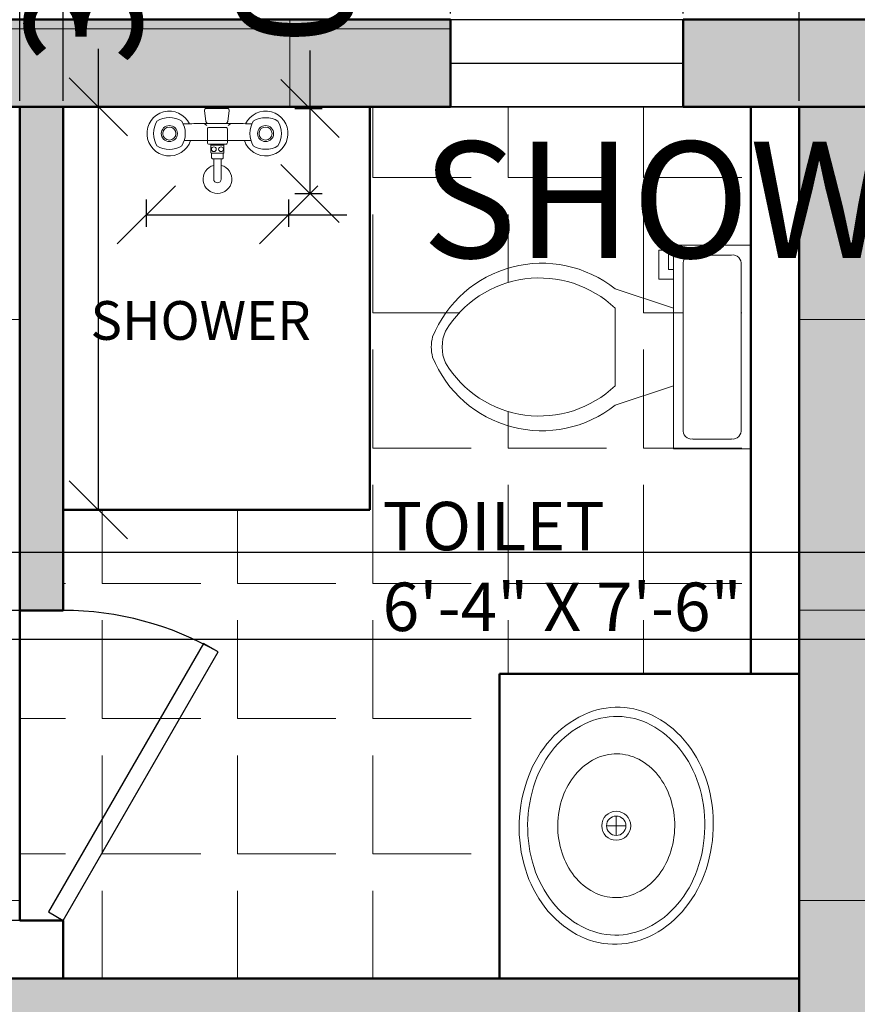
# Model space of a CAD drawing. Units: inches. Extents: x 2371 to 3019, y 129 to 700.
# Tile 6 of 14: x 2492 to 2579, y 529 to 631. Entities that reach past the tile are written whole.
import ezdxf

# ---------------------------------------------------------------- set-up
doc = ezdxf.new("R2010")
doc.units = ezdxf.units.IN
for name, color, linetype, lineweight in [('A-ANNO-DIMS', 2, 'Continuous', 18), ('A-AREA-IDEN', 7, 'Continuous', 25), ('A-DOOR', 4, 'Continuous', 25), ('A-FLOR-FIXT', 8, 'Continuous', 18), ('A-FLOR-PATT', 252, 'Continuous', 13), ('A-FURN', 8, 'Continuous', 18), ('A-GLAZ', 4, 'Continuous', 25), ('A-WALL', 7, 'Continuous', 50), ('A-WALL-PATT', 8, 'Continuous', 13)]:
    doc.layers.add(name, color=color, linetype=linetype, lineweight=lineweight)
doc.styles.get("Standard").update_dxf_attribs({"font": 'arial.ttf'})
doc.dimstyles.new('ISO-25', dxfattribs={"dimtxt": 12, "dimasz": 6, "dimexe": 1.25, "dimexo": 0.625, "dimtad": 0, "dimdec": 1, "dimlunit": 3, "dimtxsty": 'Standard', "dimblk": 'OBLIQUE', "dimblk1": 'ORIGIN2', "dimblk2": 'OBLIQUE', "dimcen": 2.5, "dimadec": 0, "dimazin": 0, "dimtfac": 1, "dimtdec": 1, "dimtmove": 0, "dimatfit": 3, "dimldrblk": 'OBLIQUE', "dimfxl": 1, "dimarcsym": 0})

# ---------------------------------------------------------------- blocks, each defined once
blk = doc.blocks.new('*U3')
for p, q in [((0, 0), (0, -6)), ((-32, 0), (-32, -6))]:
    blk.add_line(p, q)
blk.add_lwpolyline([(0, 0), (-27.71, 16), (-28.59, 14.48), (-0.88, -1.52)], close=True)
blk.add_arc((0, 0), 32, 150, 180)
blk = doc.blocks.new('Toilet - top')
for p, q in [((9.5, -6), (9.5, -2)), ((-8, -8.5), (-8, -8)), ((-7, -8), (-7, -9.5)), ((-4, -8), (-6, -14)), ((4, -8), (6, -14)), ((-10, -8.5), (-8, -8.5)), ((-10, -9.5), (-10, -8.5)), ((-7, -9.5), (-10, -9.5)), ((4, -14), (-4, -14))]:
    blk.add_line(p, q)
blk.add_lwpolyline([(10.5, -8), (10.5, 0), (-10.5, 0), (-10.5, -8)], close=True)
for points in [[(8.5, -1), (-8.5, -1)], [(-9.5, -2), (-9.5, -6)], [(-8.5, -7), (8.5, -7)]]:
    blk.add_lwpolyline(points)
for centre, radius, start, end in [((-8.62, -1.88), 0.884, 81.8699, 188.1301), ((8.62, -1.88), 0.884, 351.8699, 98.1301), ((-8.62, -6.12), 0.884, 171.8699, 278.1301), ((8.62, -6.12), 0.884, 261.8699, 8.1301), ((3.52, -21.58), 12.17, 141.4691, 247.9714), ((4.2, -21.82), 11.33, 136.3677, 238.9468), ((-3.52, -21.58), 12.17, 292.0284, 38.5307), ((-4.2, -21.82), 11.33, 301.053, 43.6321), ((0, -27.88), 4, 245.7318, 294.2682), ((0, -29), 4, 254.8605, 285.1395)]:
    blk.add_arc(centre, radius, start, end)
blk = doc.blocks.new('Sink - Oval top')
for p, q in [((-1, 0), (1, 0)), ((0, 1), (0, -1))]:
    blk.add_line(p, q)
for points in [[(-12.23, 0.39, 0.117634), (-11.46, -3.36, 0.104469), (-8.88, -6.8, 0.090016), (-5.08, -9.07, 0.08192), (-0.32, -10.02, 0.08192), (4.49, -9.38, 0.090016), (8.42, -7.36, 0.104469), (11.22, -4.09, 0.117634), (12.23, -0.39, 0.117634), (11.46, 3.36, 0.104469), (8.88, 6.8, 0.090016), (5.08, 9.07, 0.08192), (0.32, 10.02, 0.08192), (-4.49, 9.38, 0.090016), (-8.42, 7.36, 0.104469), (-11.22, 4.09, 0.117634)], [(-11.29, 0.16, 0.118622), (-10.52, -3.25, 0.104678), (-8.07, -6.36, 0.089562), (-4.54, -8.37, 0.081185), (-0.13, -9.15, 0.081185), (4.3, -8.49, 0.089562), (7.89, -6.58, 0.104678), (10.42, -3.55, 0.118622), (11.29, -0.16, 0.118622), (10.52, 3.25, 0.104678), (8.07, 6.36, 0.089562), (4.54, 8.37, 0.081185), (0.13, 9.15, 0.081185), (-4.3, 8.49, 0.089562), (-7.89, 6.58, 0.104678), (-10.42, 3.55, 0.118622)], [(-7.42, 0.08, 0.118283), (-6.91, -2.17, 0.104607), (-5.29, -4.21, 0.089718), (-2.97, -5.53, 0.081436), (-0.07, -6.04, 0.081436), (2.84, -5.59, 0.089718), (5.2, -4.33, 0.104607), (6.86, -2.32, 0.118283), (7.42, -0.08, 0.118283), (6.91, 2.17, 0.104607), (5.29, 4.21, 0.089718), (2.97, 5.53, 0.081436), (0.07, 6.04, 0.081436), (-2.84, 5.59, 0.089718), (-5.2, 4.33, 0.104607), (-6.86, 2.32, 0.118283)]]:
    blk.add_lwpolyline(points, format="xyb", close=True)
for radius in [1.5, 1]:
    blk.add_circle((0, 0), radius)
blk = doc.blocks.new('_Oblique')
at = {"color": 0, "linetype": 'ByBlock', "lineweight": -2}
blk.add_line((-0.5, -0.5), (0.5, 0.5), dxfattribs=at)
blk = doc.blocks.new('*D14')
at = {"layer": 'A-ANNO-DIMS', "color": 0, "lineweight": -2, "transparency": 16777216}
for p, q in [((2407.11, 631.6), (2407.11, 649.37)), ((2923.11, 631.6), (2923.11, 649.37)), ((2407.11, 648.12), (2643.63, 648.12)), ((2923.11, 648.12), (2686.58, 648.12))]:
    blk.add_line(p, q, dxfattribs=at)
at = {"layer": 'Defpoints', "color": 0, "lineweight": 25, "transparency": 16777216}
for p in [(2923.11, 648.12), (2407.11, 630.98), (2923.11, 630.98)]:
    blk.add_point(p, dxfattribs=at)
at = {"layer": 'A-ANNO-DIMS', "color": 0, "lineweight": -2, "transparency": 16777216, "xscale": 6, "yscale": 6, "zscale": 6, "rotation": 180}
blk.add_blockref('_Oblique', (2407.11, 648.12), dxfattribs=at)
at = {"layer": 'A-ANNO-DIMS', "color": 0, "lineweight": -2, "transparency": 16777216, "xscale": 6, "yscale": 6, "zscale": 6}
blk.add_blockref('_Oblique', (2923.11, 648.12), dxfattribs=at)
at = {"layer": 'A-ANNO-DIMS', "color": 0, "transparency": 16777216, "insert": (2665.11, 648.12), "char_height": 12, "width": 20.8486, "attachment_point": 5}
blk.add_mtext('43\'-0"', dxfattribs=at)
blk = doc.blocks.new('_Origin2')
at = {"color": 0, "linetype": 'ByBlock', "lineweight": -2}
blk.add_line((-0.5, 0), (-1, 0), dxfattribs=at)
for radius in [0.5, 0.25]:
    blk.add_circle((0, 0), radius, dxfattribs=at)
blk = doc.blocks.new('SHOWER-MIXER')
for points in [[(2511.46, 620.27), (2511.32, 620.45), (2511.19, 621.61, -0.472691), (2511.38, 621.8)], [(2513.47, 620.27), (2513.61, 620.45), (2513.75, 621.61, 0.472691), (2513.56, 621.8)], [(2506.28, 620.5, 0.281574), (2506.28, 617.95, 3.55146)], [(2508.84, 620.5, 0.281574), (2506.28, 620.5, 3.55146)], [(2508.84, 617.95, 0.281574), (2508.84, 620.5, 3.55146)], [(2508.98, 620.21, -0.00159), (2509.64, 620.23, 0.018232)], [(2509.64, 620.23, -0.004447), (2511.46, 620.27, -0.00338)], [(2511.46, 620.27, -0.000907), (2511.84, 620.27, -0.00338), (2513.23, 620.27, -0.000601), (2513.47, 620.27, 0.018232)], [(2513.47, 620.27, -0.004754), (2515.42, 620.24, 0.018232)], [(2515.42, 620.24, -0.00159), (2516.08, 620.22, 0.018232)], [(2516.23, 617.95, -0.281574), (2516.23, 620.5, -3.55146)], [(2516.23, 620.5, -0.281574), (2518.78, 620.5, -3.55146)], [(2518.78, 620.5, -0.281574), (2518.78, 617.95, -3.55146)], [(2511.5, 618.49), (2511.5, 619.7, -0.414214), (2511.66, 619.86), (2512.53, 619.86)], [(2513.56, 618.49), (2513.56, 619.7, 0.414214), (2513.4, 619.86), (2512.53, 619.86)], [(2511.5, 618.28), (2511.5, 618.49, -0.414214)], [(2511.86, 618.13), (2511.66, 618.13, -0.414214), (2511.5, 618.28)], [(2511.86, 618.13), (2511.86, 617.24, 0.414214), (2511.92, 617.18), (2511.93, 617.18)], [(2512.53, 618.13), (2511.86, 618.13, -0.414214)], [(2512.53, 618.13), (2513.2, 618.13, 0.414214)], [(2513.2, 618.13), (2513.2, 617.24, -0.414214), (2513.14, 617.18), (2513.13, 617.18)], [(2513.2, 618.13), (2513.4, 618.13, 0.414214), (2513.56, 618.28)], [(2513.56, 618.28), (2513.56, 618.49, 0.414214)], [(2506.28, 617.95, 0.281574), (2508.84, 617.95, 3.55146)], [(2511.93, 617.18), (2511.93, 616.73, 0.414214), (2512.06, 616.6), (2512.09, 616.6), (2512.14, 616.6)], [(2513.13, 617.18), (2513.13, 616.73, -0.414214), (2513.01, 616.6), (2512.98, 616.6), (2512.92, 616.6)], [(2518.78, 617.95, -0.281574), (2516.23, 617.95, -3.55146)], [(2512.14, 616.6), (2512.14, 615.94, 1)], [(2512.14, 615.94), (2512.14, 614.51, 1), (2512.92, 614.51), (2512.92, 615.94)]]:
    blk.add_lwpolyline(points, format="xyb")
for points in [[(2511.38, 621.8), (2512.47, 621.8)], [(2513.56, 621.8), (2512.47, 621.8)], [(2511.15, 620.27), (2511.42, 620.04)], [(2513.92, 620.27), (2513.64, 620.04)], [(2509.08, 618.49), (2509.75, 618.49)], [(2509.75, 618.49), (2511.5, 618.49)], [(2511.5, 618.49), (2513.56, 618.49)], [(2513.56, 618.49), (2515.31, 618.49)], [(2515.31, 618.49), (2515.98, 618.49)], [(2511.86, 618.01), (2512.53, 618.01)], [(2511.93, 617.18), (2512.53, 617.18)], [(2513.21, 618.01), (2512.53, 618.01)], [(2513.13, 617.18), (2512.53, 617.18)], [(2512.14, 616.6), (2512.53, 616.6)], [(2512.92, 616.6), (2512.53, 616.6)], [(2512.92, 615.94), (2512.92, 616.6)]]:
    blk.add_lwpolyline(points)
for centre, radius in [((2507.56, 619.22), 0.83), ((2507.56, 619.22), 0.674), ((2517.5, 619.22), 0.83), ((2517.5, 619.22), 0.674), ((2512.16, 617.6), 0.25), ((2512.9, 617.6), 0.25)]:
    blk.add_circle(centre, radius)
for centre, radius, start, end in [((2507.56, 619.22), 2.31, 25.9781, 341.5868), ((2517.5, 619.22), 2.31, 198.4132, 154.0219), ((2512.53, 614.51), 1.48, 105.2575, 74.7425)]:
    blk.add_arc(centre, radius, start, end)
blk = doc.blocks.new('*D30')
at = {"layer": 'A-ANNO-DIMS', "color": 0, "lineweight": -2, "transparency": 16777216}
for p, q in [((2505.18, 612.41), (2505.18, 609.58)), ((2519.88, 612.41), (2519.88, 609.58)), ((2505.18, 610.83), (2519.88, 610.83)), ((2519.88, 610.83), (2525.88, 610.83))]:
    blk.add_line(p, q, dxfattribs=at)
at = {"layer": 'Defpoints', "color": 0, "lineweight": 25, "transparency": 16777216}
for p in [(2505.18, 613.03), (2519.88, 613.03), (2519.88, 610.83)]:
    blk.add_point(p, dxfattribs=at)
at = {"layer": 'A-ANNO-DIMS', "color": 0, "lineweight": -2, "transparency": 16777216, "xscale": 6, "yscale": 6, "zscale": 6, "rotation": 180}
blk.add_blockref('_Oblique', (2505.18, 610.83), dxfattribs=at)
at = {"layer": 'A-ANNO-DIMS', "color": 0, "lineweight": -2, "transparency": 16777216, "xscale": 6, "yscale": 6, "zscale": 6}
blk.add_blockref('_Oblique', (2519.88, 610.83), dxfattribs=at)
at = {"layer": 'A-ANNO-DIMS', "color": 0, "transparency": 16777216, "insert": (2645.95, 610.83), "char_height": 12, "attachment_point": 5}
blk.add_mtext('SHOWER MIXER 1\'-2 1/2" TYP.', dxfattribs=at)
blk = doc.blocks.new('*D31')
at = {"layer": 'A-ANNO-DIMS', "color": 0, "lineweight": -2, "transparency": 16777216}
for p, q in [((2522.09, 621.8), (2522.09, 627.8)), ((2520.51, 621.8), (2523.34, 621.8)), ((2522.09, 613.03), (2522.09, 621.8)), ((2520.51, 613.03), (2523.34, 613.03))]:
    blk.add_line(p, q, dxfattribs=at)
at = {"layer": 'Defpoints', "color": 0, "lineweight": 25, "transparency": 16777216}
for p in [(2519.88, 621.8), (2522.09, 621.8), (2519.88, 613.03)]:
    blk.add_point(p, dxfattribs=at)
at = {"layer": 'A-ANNO-DIMS', "color": 0, "lineweight": -2, "transparency": 16777216, "xscale": 6, "yscale": 6, "zscale": 6}
for p, rotation in [((2522.09, 621.8), 90), ((2522.09, 613.03), 270)]:
    blk.add_blockref('_Oblique', p, dxfattribs=dict(at, rotation=rotation))
at = {"layer": 'A-ANNO-DIMS', "color": 0, "transparency": 16777216, "insert": (2522.09, 665), "char_height": 12, "attachment_point": 5, "rotation": 90}
blk.add_mtext('0\'-9" TYP.', dxfattribs=at)
blk = doc.blocks.new('*D33')
at = {"layer": 'A-ANNO-DIMS', "color": 0, "lineweight": -2, "transparency": 16777216}
for p, q in [((2578.94, 508.6), (2578.94, 518.23)), ((2615.61, 508.6), (2615.61, 518.23)), ((2578.94, 516.98), (2572.94, 516.98)), ((2615.61, 516.98), (2578.94, 516.98))]:
    blk.add_line(p, q, dxfattribs=at)
at = {"layer": 'Defpoints', "color": 0, "lineweight": 25, "transparency": 16777216}
for p in [(2578.94, 516.98), (2578.94, 507.98), (2615.61, 507.98)]:
    blk.add_point(p, dxfattribs=at)
at = {"layer": 'A-ANNO-DIMS', "color": 0, "lineweight": -2, "transparency": 16777216, "xscale": 6, "yscale": 6, "zscale": 6, "rotation": 180}
blk.add_blockref('_Oblique', (2578.94, 516.98), dxfattribs=at)
at = {"layer": 'A-ANNO-DIMS', "color": 0, "lineweight": -2, "transparency": 16777216, "xscale": 6, "yscale": 6, "zscale": 6}
blk.add_blockref('_Oblique', (2615.61, 516.98), dxfattribs=at)
at = {"layer": 'A-ANNO-DIMS', "color": 0, "transparency": 16777216, "insert": (2542.39, 516.98), "char_height": 12, "attachment_point": 5}
blk.add_mtext('3\'-0 1/2"', dxfattribs=at)
blk = doc.blocks.new('*D35')
at = {"layer": 'A-ANNO-DIMS', "color": 0, "lineweight": -2, "transparency": 16777216}
for p, q in [((2416.11, 622.6), (2416.11, 660.28)), ((2492.11, 622.6), (2492.11, 660.28)), ((2416.11, 659.03), (2437.5, 659.03)), ((2492.11, 659.03), (2470.71, 659.03))]:
    blk.add_line(p, q, dxfattribs=at)
at = {"layer": 'Defpoints', "color": 0, "lineweight": 25, "transparency": 16777216}
for p in [(2492.11, 659.03), (2416.11, 621.98), (2492.11, 621.98)]:
    blk.add_point(p, dxfattribs=at)
at = {"layer": 'A-ANNO-DIMS', "color": 0, "lineweight": -2, "transparency": 16777216, "xscale": 6, "yscale": 6, "zscale": 6, "rotation": 180}
blk.add_blockref('_Oblique', (2416.11, 659.03), dxfattribs=at)
at = {"layer": 'A-ANNO-DIMS', "color": 0, "lineweight": -2, "transparency": 16777216, "xscale": 6, "yscale": 6, "zscale": 6}
blk.add_blockref('_Oblique', (2492.11, 659.03), dxfattribs=at)
at = {"layer": 'A-ANNO-DIMS', "color": 0, "transparency": 16777216, "insert": (2454.11, 659.03), "char_height": 12, "attachment_point": 5}
blk.add_mtext('6\'-4"', dxfattribs=at)
blk = doc.blocks.new('*D36')
at = {"layer": 'A-ANNO-DIMS', "color": 0, "lineweight": -2, "transparency": 16777216}
for p, q in [((2492.11, 622.6), (2492.11, 660.28)), ((2496.61, 622.6), (2496.61, 660.28)), ((2492.11, 659.03), (2496.61, 659.03)), ((2496.61, 659.03), (2502.61, 659.03))]:
    blk.add_line(p, q, dxfattribs=at)
at = {"layer": 'Defpoints', "color": 0, "lineweight": 25, "transparency": 16777216}
for p in [(2496.61, 659.03), (2492.11, 621.98), (2496.61, 621.98)]:
    blk.add_point(p, dxfattribs=at)
at = {"layer": 'A-ANNO-DIMS', "color": 0, "lineweight": -2, "transparency": 16777216, "xscale": 6, "yscale": 6, "zscale": 6, "rotation": 180}
blk.add_blockref('_Oblique', (2492.11, 659.03), dxfattribs=at)
at = {"layer": 'A-ANNO-DIMS', "color": 0, "lineweight": -2, "transparency": 16777216, "xscale": 6, "yscale": 6, "zscale": 6}
blk.add_blockref('_Oblique', (2496.61, 659.03), dxfattribs=at)
at = {"layer": 'A-ANNO-DIMS', "color": 0, "transparency": 16777216, "insert": (2533.16, 659.03), "char_height": 12, "attachment_point": 5}
blk.add_mtext('0\'-4 1/2"', dxfattribs=at)
blk = doc.blocks.new('*D37')
at = {"layer": 'A-ANNO-DIMS', "color": 0, "lineweight": -2, "transparency": 16777216}
for p, q in [((2496.61, 622.6), (2496.61, 660.28)), ((2536.61, 631.6), (2536.61, 660.28)), ((2496.61, 659.03), (2500.03, 659.03)), ((2536.61, 659.03), (2533.18, 659.03))]:
    blk.add_line(p, q, dxfattribs=at)
at = {"layer": 'Defpoints', "color": 0, "lineweight": 25, "transparency": 16777216}
for p in [(2536.61, 659.03), (2536.61, 630.98), (2496.61, 621.98)]:
    blk.add_point(p, dxfattribs=at)
at = {"layer": 'A-ANNO-DIMS', "color": 0, "lineweight": -2, "transparency": 16777216, "xscale": 6, "yscale": 6, "zscale": 6, "rotation": 180}
blk.add_blockref('_Oblique', (2496.61, 659.03), dxfattribs=at)
at = {"layer": 'A-ANNO-DIMS', "color": 0, "lineweight": -2, "transparency": 16777216, "xscale": 6, "yscale": 6, "zscale": 6}
blk.add_blockref('_Oblique', (2536.61, 659.03), dxfattribs=at)
at = {"layer": 'A-ANNO-DIMS', "color": 0, "transparency": 16777216, "insert": (2516.61, 659.03), "char_height": 12, "attachment_point": 5}
blk.add_mtext('3\'-4"', dxfattribs=at)
blk = doc.blocks.new('*D39')
at = {"layer": 'A-ANNO-DIMS', "color": 0, "lineweight": -2, "transparency": 16777216}
for p, q in [((2560.61, 631.6), (2560.61, 660.28)), ((2572.61, 622.6), (2572.61, 660.28)), ((2560.61, 659.03), (2572.61, 659.03)), ((2572.61, 659.03), (2578.61, 659.03))]:
    blk.add_line(p, q, dxfattribs=at)
at = {"layer": 'Defpoints', "color": 0, "lineweight": 25, "transparency": 16777216}
for p in [(2572.61, 659.03), (2560.61, 630.98), (2572.61, 621.98)]:
    blk.add_point(p, dxfattribs=at)
at = {"layer": 'A-ANNO-DIMS', "color": 0, "lineweight": -2, "transparency": 16777216, "xscale": 6, "yscale": 6, "zscale": 6, "rotation": 180}
blk.add_blockref('_Oblique', (2560.61, 659.03), dxfattribs=at)
at = {"layer": 'A-ANNO-DIMS', "color": 0, "lineweight": -2, "transparency": 16777216, "xscale": 6, "yscale": 6, "zscale": 6}
blk.add_blockref('_Oblique', (2572.61, 659.03), dxfattribs=at)
at = {"layer": 'A-ANNO-DIMS', "color": 0, "transparency": 16777216, "insert": (2594.61, 659.03), "char_height": 12, "attachment_point": 5}
blk.add_mtext('1\'-0"', dxfattribs=at)
blk = doc.blocks.new('*D40')
at = {"layer": 'A-ANNO-DIMS', "color": 0, "lineweight": -2, "transparency": 16777216}
for p, q in [((2572.61, 622.6), (2572.61, 660.28)), ((2581.61, 622.6), (2581.61, 660.28)), ((2572.61, 659.03), (2581.61, 659.03)), ((2581.61, 659.03), (2587.61, 659.03))]:
    blk.add_line(p, q, dxfattribs=at)
at = {"layer": 'Defpoints', "color": 0, "lineweight": 25, "transparency": 16777216}
for p in [(2581.61, 659.03), (2572.61, 621.98), (2581.61, 621.98)]:
    blk.add_point(p, dxfattribs=at)
at = {"layer": 'A-ANNO-DIMS', "color": 0, "lineweight": -2, "transparency": 16777216, "xscale": 6, "yscale": 6, "zscale": 6, "rotation": 180}
blk.add_blockref('_Oblique', (2572.61, 659.03), dxfattribs=at)
at = {"layer": 'A-ANNO-DIMS', "color": 0, "lineweight": -2, "transparency": 16777216, "xscale": 6, "yscale": 6, "zscale": 6}
blk.add_blockref('_Oblique', (2581.61, 659.03), dxfattribs=at)
at = {"layer": 'A-ANNO-DIMS', "color": 0, "transparency": 16777216, "insert": (2604.18, 659.03), "char_height": 12, "attachment_point": 5}
blk.add_mtext('0\'-9"', dxfattribs=at)
blk = doc.blocks.new('*D65')
at = {"layer": 'A-ANNO-DIMS', "color": 0, "lineweight": -2, "transparency": 16777216}
for p, q in [((2618.98, 621.98), (2377.81, 621.98)), ((2379.06, 621.98), (2379.06, 620.21)), ((2379.06, 575.98), (2379.06, 577.74)), ((2616.98, 575.98), (2377.81, 575.98))]:
    blk.add_line(p, q, dxfattribs=at)
at = {"layer": 'Defpoints', "color": 0, "lineweight": 25, "transparency": 16777216}
for p in [(2379.06, 621.98), (2619.61, 621.98), (2617.61, 575.98)]:
    blk.add_point(p, dxfattribs=at)
at = {"layer": 'A-ANNO-DIMS', "color": 0, "lineweight": -2, "transparency": 16777216, "xscale": 6, "yscale": 6, "zscale": 6}
for p, rotation in [((2379.06, 621.98), 90), ((2379.06, 575.98), 270)]:
    blk.add_blockref('_Oblique', p, dxfattribs=dict(at, rotation=rotation))
at = {"layer": 'A-ANNO-DIMS', "color": 0, "transparency": 16777216, "insert": (2379.06, 598.98), "char_height": 12, "attachment_point": 5, "rotation": 90}
blk.add_mtext('3\'-10"', dxfattribs=at)
blk = doc.blocks.new('*D67')
at = {"layer": 'A-ANNO-DIMS', "color": 0, "lineweight": -2, "transparency": 16777216}
for p, q in [((2379.06, 575.98), (2379.06, 581.98)), ((2616.98, 575.98), (2377.81, 575.98)), ((2379.06, 566.98), (2379.06, 575.98)), ((2616.98, 566.98), (2377.81, 566.98))]:
    blk.add_line(p, q, dxfattribs=at)
at = {"layer": 'Defpoints', "color": 0, "lineweight": 25, "transparency": 16777216}
for p in [(2379.06, 575.98), (2617.61, 575.98), (2617.61, 566.98)]:
    blk.add_point(p, dxfattribs=at)
at = {"layer": 'A-ANNO-DIMS', "color": 0, "lineweight": -2, "transparency": 16777216, "xscale": 6, "yscale": 6, "zscale": 6}
for p, rotation in [((2379.06, 575.98), 90), ((2379.06, 566.98), 270)]:
    blk.add_blockref('_Oblique', p, dxfattribs=dict(at, rotation=rotation))
at = {"layer": 'A-ANNO-DIMS', "color": 0, "transparency": 16777216, "insert": (2379.06, 598.55), "char_height": 12, "attachment_point": 5, "rotation": 90}
blk.add_mtext('0\'-9"', dxfattribs=at)
blk = doc.blocks.new('*D74')
at = {"layer": 'A-ANNO-DIMS', "color": 0, "lineweight": -2, "transparency": 16777216}
for p, q in [((2464.06, 569.98), (2464.06, 575.98)), ((2491.48, 569.98), (2462.81, 569.98)), ((2464.06, 537.98), (2464.06, 569.98)), ((2491.48, 537.98), (2462.81, 537.98))]:
    blk.add_line(p, q, dxfattribs=at)
at = {"layer": 'Defpoints', "color": 0, "lineweight": 25, "transparency": 16777216}
for p in [(2464.06, 569.98), (2492.11, 569.98), (2492.11, 537.98)]:
    blk.add_point(p, dxfattribs=at)
at = {"layer": 'A-ANNO-DIMS', "color": 0, "lineweight": -2, "transparency": 16777216, "xscale": 6, "yscale": 6, "zscale": 6}
for p, rotation in [((2464.06, 569.98), 90), ((2464.06, 537.98), 270)]:
    blk.add_blockref('_Oblique', p, dxfattribs=dict(at, rotation=rotation))
at = {"layer": 'A-ANNO-DIMS', "color": 0, "transparency": 16777216, "insert": (2464.06, 592.65), "char_height": 12, "attachment_point": 5, "rotation": 90}
blk.add_mtext('2\'-8"', dxfattribs=at)
blk = doc.blocks.new('*D78')
at = {"layer": 'A-ANNO-DIMS', "color": 0, "lineweight": -2, "transparency": 16777216}
for p, q in [((2500.23, 621.98), (2500.23, 627.98)), ((2527.66, 621.98), (2498.98, 621.98)), ((2500.23, 580.36), (2500.23, 621.98)), ((2527.66, 580.36), (2498.98, 580.36))]:
    blk.add_line(p, q, dxfattribs=at)
at = {"layer": 'Defpoints', "color": 0, "lineweight": 25, "transparency": 16777216}
for p in [(2500.23, 621.98), (2528.28, 621.98), (2528.28, 580.36)]:
    blk.add_point(p, dxfattribs=at)
at = {"layer": 'A-ANNO-DIMS', "color": 0, "lineweight": -2, "transparency": 16777216, "xscale": 6, "yscale": 6, "zscale": 6}
for p, rotation in [((2500.23, 621.98), 90), ((2500.23, 580.36), 270)]:
    blk.add_blockref('_Oblique', p, dxfattribs=dict(at, rotation=rotation))
at = {"layer": 'A-ANNO-DIMS', "color": 0, "transparency": 16777216, "insert": (2500.23, 658.53), "char_height": 12, "attachment_point": 5, "rotation": 90}
blk.add_mtext('3\'-5 1/2"', dxfattribs=at)

msp = doc.modelspace()

# ---------------------------------------------------------------- hatches: boundary and pattern name
at = {"layer": 'A-FLOR-PATT'}
h = msp.add_hatch(dxfattribs=at)
h.set_pattern_fill('_USER', color=256, scale=30, pattern_type=0)
h.set_pattern_definition([(0, (0, 0), (0, 30), [])])
h.paths.add_polyline_path([(2913.11, 498.98), (2827.61, 498.98), (2827.61, 531.98), (2832.11, 531.98), (2832.11, 537.98), (2833.61, 537.98), (2833.61, 605.98), (2818.35, 605.98, -1), (2796.86, 605.98), (2781.61, 605.98), (2781.61, 603.98), (2781.61, 533.98), (2757.61, 533.98), (2757.61, 531.98), (2797.61, 531.98), (2797.61, 522.98), (2757.61, 522.98), (2757.61, 516.98), (2754.59, 516.98), (2772.52, 485.76), (2771.01, 484.89), (2770.98, 484.93, -0.097552), (2757.61, 481.1), (2757.61, 422.48), (2837.61, 422.48), (2837.61, 362.48), (2757.61, 362.48), (2757.61, 303.98), (2835.86, 303.98, -0.09439), (2793.86, 311.98), (2793.86, 337.98), (2799.86, 337.98), (2799.86, 336.42), (2871.86, 336.42), (2871.86, 337.98), (2877.86, 337.98), (2877.86, 311.98, -0.09439), (2835.86, 303.98), (2913.11, 303.98), (2913.11, 383.18), (2904.11, 383.18), (2904.11, 419.18), (2913.11, 419.18)])
h.paths.add_polyline_path([(2788.88, 332.88), (2788.88, 308.88), (2764.88, 308.88), (2764.88, 332.88)], flags=16)
h.paths.add_polyline_path([(2788.4, 325.04, -1), (2774.4, 325.04, -1)], flags=0)
h.paths.add_polyline_path([(2781.4, 328.04), (2784.4, 325.04), (2781.4, 322.04), (2778.4, 325.04)], flags=0)
h.paths.add_polyline_path([(2782.4, 325.04, -1), (2780.4, 325.04, -1)], flags=0)
h.paths.add_polyline_path([(2748.61, 480.99), (2754.51, 480.98, 0.119303), (2770.98, 484.93), (2753.07, 516.1), (2754.59, 516.98), (2748.61, 516.98), (2748.61, 539.98), (2712.61, 539.98), (2665.11, 539.98, -0.09439), (2707.11, 531.98), (2707.11, 505.98), (2701.11, 505.98), (2701.11, 507.53), (2629.11, 507.53), (2629.11, 505.98), (2623.11, 505.98), (2623.11, 531.98, -0.09439), (2665.11, 539.98), (2581.61, 539.98), (2581.61, 522.98), (2581.61, 477.98, -0.131044), (2589.61, 507.98), (2615.61, 507.98), (2615.61, 501.98), (2614.05, 501.98), (2614.05, 453.98), (2615.61, 453.98), (2615.61, 447.98), (2589.61, 447.98, -0.131044), (2581.61, 477.98), (2581.61, 432.98), (2572.61, 432.98, 0.119303), (2556.14, 428.99), (2574.12, 397.85), (2572.61, 396.98), (2578.61, 396.98), (2581.61, 396.98), (2581.61, 390.98), (2748.61, 390.98)])
h.paths.add_polyline_path([(2683.1, 447.25), (2652.43, 447.25), (2652.43, 492.22), (2683.1, 492.22)], flags=16)
h.paths.add_polyline_path([(2682.1, 448.25), (2653.43, 448.25), (2653.43, 491.22), (2682.1, 491.22)], flags=0)
h.paths.add_polyline_path([(2613.58, 512.06), (2589.58, 512.06), (2589.58, 536.06), (2613.58, 536.06)], flags=16)
h.paths.add_polyline_path([(2599.1, 528.22, -1), (2613.1, 528.22, -1)], flags=0)
h.paths.add_polyline_path([(2609.1, 528.22), (2606.1, 525.22), (2603.1, 528.22), (2606.1, 531.22)], flags=0)
h.paths.add_polyline_path([(2607.1, 528.22, -1), (2605.1, 528.22, -1)], flags=0)
h.paths.add_polyline_path([(2581.61, 522.98), (2581.61, 621.98), (2572.61, 621.98), (2572.61, 522.98), (2572.61, 500.98), (2565.85, 500.98), (2565.85, 500.15), (2564.82, 500.15), (2561.16, 500.19), (2561.16, 500.17), (2560.13, 500.3), (2560.22, 500.98), (2556.38, 500.98), (2556.43, 500.22), (2555.4, 500.14), (2555.34, 500.98), (2551.07, 500.98), (2551.07, 500.15), (2550.04, 500.15), (2547.64, 500.19), (2547.64, 500.15), (2546.61, 500.15), (2541.79, 500.22), (2540.72, 500.13), (2540.65, 500.98), (2533.37, 500.98), (2533.37, 500.15), (2532.34, 500.15), (2529.13, 500.21), (2529.12, 500.13), (2528.09, 500.22), (2528.16, 500.98), (2523.23, 500.98), (2523.23, 500.15), (2522.2, 500.15), (2519.8, 500.21), (2519.8, 500.15), (2518.77, 500.15), (2514.45, 500.26), (2514.44, 500.14), (2513.41, 500.22), (2513.47, 500.98), (2509.62, 500.98), (2509.71, 500.3), (2508.69, 500.17), (2508.58, 500.98), (2505.03, 500.98), (2505.03, 500.15), (2503.99, 500.15), (2501.07, 500.29), (2501.07, 500.15), (2500.04, 500.15), (2496.44, 500.37), (2496.44, 500.15), (2495.4, 500.15), (2492.55, 500.41), (2492.18, 500.35), (2492.09, 500.98), (2486.11, 500.98), (2486.11, 524.98), (2486.11, 531.98), (2490.61, 531.98), (2490.61, 537.98), (2492.11, 537.98), (2492.11, 605.98), (2476.85, 605.98, -1), (2455.36, 605.98), (2440.11, 605.98), (2440.11, 533.98), (2416.11, 533.98), (2416.11, 605.98), (2416.11, 621.98), (2536.61, 621.98), (2536.61, 630.98), (2407.11, 630.98), (2407.11, 363.98), (2416.11, 363.98), (2416.11, 431.48), (2496.11, 431.48), (2496.11, 371.48), (2416.11, 371.48), (2416.11, 303.98), (2494.36, 303.98, -0.09439), (2452.36, 311.98), (2452.36, 337.98), (2458.36, 337.98), (2458.36, 336.42), (2530.36, 336.42), (2530.36, 337.98), (2536.36, 337.98), (2536.36, 311.98, -0.09439), (2494.36, 303.98), (2572.61, 303.98), (2572.61, 381.98), (2572.61, 396.98), (2554.61, 428.15), (2556.12, 429.03), (2556.14, 428.99, -0.119303), (2572.61, 432.98), (2578.61, 432.98), (2581.61, 432.98)])
h.paths.add_polyline_path([(2450.11, 500.98), (2444.5, 500.98), (2444.44, 500.14), (2443.41, 500.22), (2443.47, 500.98), (2439.62, 500.98), (2439.71, 500.3), (2438.69, 500.17), (2438.58, 500.98), (2435.02, 500.98), (2435.02, 500.15), (2433.99, 500.15), (2433.99, 500.98), (2431.07, 500.98), (2431.07, 500.15), (2430.04, 500.15), (2430.04, 500.98), (2426.43, 500.98), (2426.43, 500.15), (2425.4, 500.15), (2425.4, 500.98), (2423.13, 500.98), (2423.2, 500.5), (2422.18, 500.35), (2422.09, 500.98), (2416.11, 500.98), (2416.11, 524.98), (2416.11, 531.98), (2450.11, 531.98), (2450.11, 522.98)], flags=16)
h.paths.add_polyline_path([(2449.11, 501.98), (2417.11, 501.98), (2417.11, 522.98), (2417.11, 523.98), (2449.11, 523.98)], flags=0)
h.paths.add_polyline_path([(2420.7, 510.73), (2419.36, 520.07), (2420.38, 520.22), (2421.74, 510.73), (2425.4, 510.73), (2425.4, 520.07), (2426.43, 520.07), (2426.43, 510.73), (2430.04, 510.73), (2430.04, 520.07), (2431.07, 520.07), (2431.07, 510.73), (2433.99, 510.73), (2433.99, 520.07), (2435.02, 520.07), (2435.02, 510.73), (2437.35, 510.73), (2436.18, 519.93), (2437.2, 520.06), (2438.39, 510.73), (2444.17, 510.73), (2444.85, 520.08), (2445.88, 520.01), (2445.21, 510.73)], flags=0)
h.paths.add_polyline_path([(2446.94, 336.11), (2446.94, 312.11), (2422.94, 312.11), (2422.94, 336.11)], flags=16)
h.paths.add_polyline_path([(2446.46, 328.27, -1), (2432.46, 328.27, -1)], flags=0)
h.paths.add_polyline_path([(2439.46, 331.27), (2442.46, 328.27), (2439.46, 325.27), (2436.46, 328.27)], flags=0)
h.paths.add_polyline_path([(2440.46, 328.27, -1), (2438.46, 328.27, -1)], flags=0)
h.paths.add_polyline_path([(2816, 444.88), (2866.87, 444.88), (2866.87, 463.54), (2816, 463.54)], flags=24)
h.paths.add_polyline_path([(2794.21, 558.3), (2833.34, 558.3), (2833.34, 576.96), (2794.21, 576.96)], flags=24)
h.paths.add_polyline_path([(2651.69, 411.53), (2711.04, 411.53), (2711.04, 430.19), (2651.69, 430.19)], flags=24)
h.paths.add_polyline_path([(2494.09, 444.88), (2544.97, 444.88), (2544.97, 463.54), (2494.09, 463.54)], flags=24)
h.paths.add_polyline_path([(2444.55, 565.02), (2483.69, 565.02), (2483.69, 583.68), (2444.55, 583.68)], flags=24)
h = msp.add_hatch(dxfattribs=at)
h.set_pattern_fill('_USER', color=256, scale=30, angle=90, pattern_type=0)
h.set_pattern_definition([(90, (0, 0), (-30, 2e-15), [])])
h.paths.add_polyline_path([(2913.11, 498.98), (2827.61, 498.98), (2827.61, 531.98), (2832.11, 531.98), (2832.11, 537.98), (2833.61, 537.98), (2833.61, 605.98), (2818.35, 605.98, -1), (2796.86, 605.98), (2781.61, 605.98), (2781.61, 603.98), (2781.61, 533.98), (2757.61, 533.98), (2757.61, 531.98), (2797.61, 531.98), (2797.61, 522.98), (2757.61, 522.98), (2757.61, 516.98), (2754.59, 516.98), (2772.52, 485.76), (2771.01, 484.89), (2770.98, 484.93, -0.097552), (2757.61, 481.1), (2757.61, 422.48), (2837.61, 422.48), (2837.61, 362.48), (2757.61, 362.48), (2757.61, 303.98), (2835.86, 303.98, -0.09439), (2793.86, 311.98), (2793.86, 337.98), (2799.86, 337.98), (2799.86, 336.42), (2871.86, 336.42), (2871.86, 337.98), (2877.86, 337.98), (2877.86, 311.98, -0.09439), (2835.86, 303.98), (2913.11, 303.98), (2913.11, 383.18), (2904.11, 383.18), (2904.11, 419.18), (2913.11, 419.18)])
h.paths.add_polyline_path([(2788.88, 332.88), (2788.88, 308.88), (2764.88, 308.88), (2764.88, 332.88)], flags=16)
h.paths.add_polyline_path([(2788.4, 325.04, -1), (2774.4, 325.04, -1)], flags=0)
h.paths.add_polyline_path([(2781.4, 328.04), (2784.4, 325.04), (2781.4, 322.04), (2778.4, 325.04)], flags=0)
h.paths.add_polyline_path([(2782.4, 325.04, -1), (2780.4, 325.04, -1)], flags=0)
h.paths.add_polyline_path([(2748.61, 480.99), (2754.51, 480.98, 0.119303), (2770.98, 484.93), (2753.07, 516.1), (2754.59, 516.98), (2748.61, 516.98), (2748.61, 539.98), (2712.61, 539.98), (2665.11, 539.98, -0.09439), (2707.11, 531.98), (2707.11, 505.98), (2701.11, 505.98), (2701.11, 507.53), (2629.11, 507.53), (2629.11, 505.98), (2623.11, 505.98), (2623.11, 531.98, -0.09439), (2665.11, 539.98), (2581.61, 539.98), (2581.61, 522.98), (2581.61, 477.98, -0.131044), (2589.61, 507.98), (2615.61, 507.98), (2615.61, 501.98), (2614.05, 501.98), (2614.05, 453.98), (2615.61, 453.98), (2615.61, 447.98), (2589.61, 447.98, -0.131044), (2581.61, 477.98), (2581.61, 432.98), (2572.61, 432.98, 0.119303), (2556.14, 428.99), (2574.12, 397.85), (2572.61, 396.98), (2578.61, 396.98), (2581.61, 396.98), (2581.61, 390.98), (2748.61, 390.98)])
h.paths.add_polyline_path([(2683.1, 447.25), (2652.43, 447.25), (2652.43, 492.22), (2683.1, 492.22)], flags=16)
h.paths.add_polyline_path([(2682.1, 448.25), (2653.43, 448.25), (2653.43, 491.22), (2682.1, 491.22)], flags=0)
h.paths.add_polyline_path([(2613.58, 512.06), (2589.58, 512.06), (2589.58, 536.06), (2613.58, 536.06)], flags=16)
h.paths.add_polyline_path([(2599.1, 528.22, -1), (2613.1, 528.22, -1)], flags=0)
h.paths.add_polyline_path([(2609.1, 528.22), (2606.1, 525.22), (2603.1, 528.22), (2606.1, 531.22)], flags=0)
h.paths.add_polyline_path([(2607.1, 528.22, -1), (2605.1, 528.22, -1)], flags=0)
h.paths.add_polyline_path([(2581.61, 522.98), (2581.61, 621.98), (2572.61, 621.98), (2572.61, 522.98), (2572.61, 500.98), (2565.85, 500.98), (2565.85, 500.15), (2564.82, 500.15), (2561.16, 500.19), (2561.16, 500.17), (2560.13, 500.3), (2560.22, 500.98), (2556.38, 500.98), (2556.43, 500.22), (2555.4, 500.14), (2555.34, 500.98), (2551.07, 500.98), (2551.07, 500.15), (2550.04, 500.15), (2547.64, 500.19), (2547.64, 500.15), (2546.61, 500.15), (2541.79, 500.22), (2540.72, 500.13), (2540.65, 500.98), (2533.37, 500.98), (2533.37, 500.15), (2532.34, 500.15), (2529.13, 500.21), (2529.12, 500.13), (2528.09, 500.22), (2528.16, 500.98), (2523.23, 500.98), (2523.23, 500.15), (2522.2, 500.15), (2519.8, 500.21), (2519.8, 500.15), (2518.77, 500.15), (2514.45, 500.26), (2514.44, 500.14), (2513.41, 500.22), (2513.47, 500.98), (2509.62, 500.98), (2509.71, 500.3), (2508.69, 500.17), (2508.58, 500.98), (2505.03, 500.98), (2505.03, 500.15), (2503.99, 500.15), (2501.07, 500.29), (2501.07, 500.15), (2500.04, 500.15), (2496.44, 500.37), (2496.44, 500.15), (2495.4, 500.15), (2492.55, 500.41), (2492.18, 500.35), (2492.09, 500.98), (2486.11, 500.98), (2486.11, 524.98), (2486.11, 531.98), (2490.61, 531.98), (2490.61, 537.98), (2492.11, 537.98), (2492.11, 605.98), (2476.85, 605.98, -1), (2455.36, 605.98), (2440.11, 605.98), (2440.11, 533.98), (2416.11, 533.98), (2416.11, 605.98), (2416.11, 621.98), (2536.61, 621.98), (2536.61, 630.98), (2407.11, 630.98), (2407.11, 363.98), (2416.11, 363.98), (2416.11, 431.48), (2496.11, 431.48), (2496.11, 371.48), (2416.11, 371.48), (2416.11, 303.98), (2494.36, 303.98, -0.09439), (2452.36, 311.98), (2452.36, 337.98), (2458.36, 337.98), (2458.36, 336.42), (2530.36, 336.42), (2530.36, 337.98), (2536.36, 337.98), (2536.36, 311.98, -0.09439), (2494.36, 303.98), (2572.61, 303.98), (2572.61, 381.98), (2572.61, 396.98), (2554.61, 428.15), (2556.12, 429.03), (2556.14, 428.99, -0.119303), (2572.61, 432.98), (2578.61, 432.98), (2581.61, 432.98)])
h.paths.add_polyline_path([(2450.11, 500.98), (2444.5, 500.98), (2444.44, 500.14), (2443.41, 500.22), (2443.47, 500.98), (2439.62, 500.98), (2439.71, 500.3), (2438.69, 500.17), (2438.58, 500.98), (2435.02, 500.98), (2435.02, 500.15), (2433.99, 500.15), (2433.99, 500.98), (2431.07, 500.98), (2431.07, 500.15), (2430.04, 500.15), (2430.04, 500.98), (2426.43, 500.98), (2426.43, 500.15), (2425.4, 500.15), (2425.4, 500.98), (2423.13, 500.98), (2423.2, 500.5), (2422.18, 500.35), (2422.09, 500.98), (2416.11, 500.98), (2416.11, 524.98), (2416.11, 531.98), (2450.11, 531.98), (2450.11, 522.98)], flags=16)
h.paths.add_polyline_path([(2449.11, 501.98), (2417.11, 501.98), (2417.11, 522.98), (2417.11, 523.98), (2449.11, 523.98)], flags=0)
h.paths.add_polyline_path([(2420.7, 510.73), (2419.36, 520.07), (2420.38, 520.22), (2421.74, 510.73), (2425.4, 510.73), (2425.4, 520.07), (2426.43, 520.07), (2426.43, 510.73), (2430.04, 510.73), (2430.04, 520.07), (2431.07, 520.07), (2431.07, 510.73), (2433.99, 510.73), (2433.99, 520.07), (2435.02, 520.07), (2435.02, 510.73), (2437.35, 510.73), (2436.18, 519.93), (2437.2, 520.06), (2438.39, 510.73), (2444.17, 510.73), (2444.85, 520.08), (2445.88, 520.01), (2445.21, 510.73)], flags=0)
h.paths.add_polyline_path([(2446.94, 336.11), (2446.94, 312.11), (2422.94, 312.11), (2422.94, 336.11)], flags=16)
h.paths.add_polyline_path([(2446.46, 328.27, -1), (2432.46, 328.27, -1)], flags=0)
h.paths.add_polyline_path([(2439.46, 331.27), (2442.46, 328.27), (2439.46, 325.27), (2436.46, 328.27)], flags=0)
h.paths.add_polyline_path([(2440.46, 328.27, -1), (2438.46, 328.27, -1)], flags=0)
h.paths.add_polyline_path([(2816, 444.88), (2866.87, 444.88), (2866.87, 463.54), (2816, 463.54)], flags=24)
h.paths.add_polyline_path([(2794.21, 558.3), (2833.34, 558.3), (2833.34, 576.96), (2794.21, 576.96)], flags=24)
h.paths.add_polyline_path([(2651.69, 411.53), (2711.04, 411.53), (2711.04, 430.19), (2651.69, 430.19)], flags=24)
h.paths.add_polyline_path([(2494.09, 444.88), (2544.97, 444.88), (2544.97, 463.54), (2494.09, 463.54)], flags=24)
h.paths.add_polyline_path([(2444.55, 565.02), (2483.69, 565.02), (2483.69, 583.68), (2444.55, 583.68)], flags=24)
h = msp.add_hatch(dxfattribs=at)
h.set_pattern_fill('ANGLE', color=256, scale=2)
h.set_pattern_definition([(0, (0, 0), (0, 13.97), [10.16, -3.81]), (90, (0, 0), (-13.97, 9e-16), [10.16, -3.81])])
h.paths.add_polyline_path([(2567.61, 621.98), (2560.61, 621.98), (2536.61, 621.98), (2528.28, 621.98), (2528.28, 580.36), (2496.61, 580.36), (2496.61, 569.98), (2492.11, 569.98), (2492.11, 537.98), (2496.61, 537.98), (2496.61, 531.98), (2541.64, 531.98), (2541.64, 563.44), (2567.61, 563.44)])
h.paths.add_polyline_path([(2536.08, 595.53, -0.215004), (2536.08, 598.82, -0.48008), (2553.61, 601.18), (2553.61, 593.18, -0.48008)], flags=16)
h.paths.add_polyline_path([(2560.61, 588.68), (2560.61, 605.68, -0.5), (2561.61, 606.68), (2565.61, 606.68, -0.5), (2566.61, 605.68), (2566.61, 588.68, -0.5), (2565.61, 587.68), (2561.61, 587.68, -0.5)], flags=16)
at = {"layer": 'A-WALL-PATT'}
h = msp.add_hatch(color=256, dxfattribs=at)
h.dxf.hatch_style = 1
h.paths.add_polyline_path([(2536.61, 630.98), (2407.11, 630.98), (2407.11, 363.98), (2416.11, 363.98), (2416.11, 498.98), (2416.11, 522.98), (2416.11, 531.98), (2416.11, 603.98), (2416.11, 621.98), (2536.61, 621.98)])
h.paths.add_polyline_path([(2630.98, 630.98), (2560.61, 630.98), (2560.61, 621.98), (2630.98, 621.98)])
h.paths.add_polyline_path([(2878.11, 630.98), (2699.23, 630.98), (2699.23, 621.98), (2878.11, 621.98)])
h.paths.add_polyline_path([(2496.61, 621.98), (2492.11, 621.98), (2492.11, 569.98), (2496.61, 569.98)], flags=17)
h.paths.add_polyline_path([(2581.61, 621.98), (2572.61, 621.98), (2572.61, 522.98), (2572.61, 498.98), (2572.61, 432.98), (2578.61, 432.98), (2581.61, 432.98), (2581.61, 522.98)])
h.paths.add_polyline_path([(2572.61, 531.98), (2486.11, 531.98), (2486.11, 522.98), (2572.61, 522.98)])
h.paths.add_polyline_path([(2450.11, 531.98), (2440.11, 531.98), (2416.11, 531.98), (2416.11, 522.98), (2450.11, 522.98)], flags=17)
h.paths.add_polyline_path([(2416.11, 315.98), (2407.11, 315.98), (2407.11, 294.98), (2458.11, 294.98), (2458.11, 303.98), (2416.11, 303.98)])
h.paths.add_polyline_path([(2757.61, 303.98), (2530.61, 303.98), (2530.61, 294.98), (2757.61, 294.98)])
h.paths.add_polyline_path([(2581.61, 381.98), (2605.61, 381.98), (2617.61, 381.98), (2617.61, 390.98), (2581.61, 390.98), (2581.61, 396.98), (2572.61, 396.98), (2572.61, 381.98), (2572.61, 303.98), (2581.61, 303.98)])
h.paths.add_polyline_path([(2757.61, 480.98), (2748.61, 480.98), (2748.61, 381.98), (2748.61, 303.98), (2757.61, 303.98), (2757.61, 381.98), (2757.61, 422.48)])
h.paths.add_polyline_path([(2797.61, 531.98), (2757.61, 531.98), (2757.61, 603.98), (2757.61, 621.98), (2748.61, 621.98), (2748.61, 516.99), (2754.59, 516.98), (2757.61, 516.98), (2757.61, 522.98), (2797.61, 522.98)])
h.paths.add_polyline_path([(2913.11, 531.98), (2827.61, 531.98), (2827.61, 522.98), (2913.11, 522.98)])
h.paths.add_polyline_path([(2923.11, 630.98), (2902.11, 630.98), (2902.11, 621.98), (2914.11, 621.98), (2914.11, 363.98), (2923.11, 363.98)])
h.paths.add_polyline_path([(2923.11, 315.98), (2914.11, 315.98), (2914.11, 303.98), (2866.11, 303.98), (2866.11, 294.98), (2923.11, 294.98)])
h.paths.add_polyline_path([(2793.61, 303.98), (2757.61, 303.98), (2757.61, 294.98), (2793.61, 294.98)])

# ---------------------------------------------------------------- linework, layer by layer
at = {"layer": 'A-FURN'}
for points in [[(2511.38, 621.8, -0.080845), (2512.47, 621.98, -0.039297)], [(2513.56, 621.8, 0.080845), (2512.47, 621.98, 0.039297)]]:
    msp.add_lwpolyline(points, format="xyb", dxfattribs=at)
at = {"layer": 'A-GLAZ', "ltscale": 0.5}
for p, q in [((2536.61, 630.98), (2560.61, 630.98)), ((2536.61, 626.48), (2560.61, 626.48)), ((2536.61, 621.98), (2560.61, 621.98))]:
    msp.add_line(p, q, dxfattribs=at)
at = {"layer": 'A-WALL'}
for p, q in [((2536.61, 630.98), (2407.11, 630.98)), ((2536.61, 630.98), (2536.61, 621.98)), ((2560.61, 630.98), (2560.61, 621.98)), ((2878.11, 630.98), (2560.61, 630.98)), ((2536.61, 621.98), (2416.11, 621.98)), ((2492.11, 621.98), (2492.11, 537.98)), ((2496.61, 621.98), (2496.61, 569.98)), ((2528.28, 621.98), (2528.28, 580.36)), ((2878.11, 621.98), (2560.61, 621.98)), ((2567.61, 621.98), (2567.61, 563.44)), ((2572.61, 621.98), (2572.61, 522.98)), ((2528.28, 580.36), (2496.61, 580.36)), ((2496.61, 569.98), (2492.11, 569.98)), ((2541.64, 531.98), (2541.64, 563.44)), ((2541.64, 563.44), (2572.61, 563.44)), ((2496.61, 537.98), (2492.11, 537.98)), ((2496.61, 537.98), (2496.61, 531.98)), ((2572.61, 531.98), (2486.11, 531.98))]:
    msp.add_line(p, q, dxfattribs=at)

# ---------------------------------------------------------------- block references
at = {"layer": 'A-DOOR', "rotation": 270}
msp.add_blockref('*U3', (2496.61, 537.98), dxfattribs=at)
at = {"layer": 'A-FLOR-FIXT'}
msp.add_blockref('SHOWER-MIXER', (0, 0), dxfattribs=at)
at = {"layer": 'A-FLOR-FIXT', "rotation": 270}
for name, p in [('Toilet - top', (2567.61, 597.18)), ('Sink - Oval top', (2553.71, 547.75))]:
    msp.add_blockref(name, p, dxfattribs=at)

# ---------------------------------------------------------------- texts
at = {"layer": 'A-AREA-IDEN', "ltscale": 2, "attachment_point": 1}
for s, insert, char_height in [('SHOWER', (2499.42, 601.92), 4), ('TOILET\\P6\'-4" X 7\'-6"', (2529.58, 581.19), 5)]:
    msp.add_mtext_dynamic_manual_height_columns(s, width=39.2097, gutter_width=12.5, heights=[0], dxfattribs=dict(at, insert=insert, char_height=char_height))

# ---------------------------------------------------------------- dimensions: what is measured, and where the dimension line sits
at = {"layer": 'A-ANNO-DIMS'}
dim = msp.add_linear_dim(base=(2522.09, 621.8), p1=(2519.88, 613.03), p2=(2519.88, 621.8), angle=90, text='<> TYP.', dimstyle='ISO-25', override={"dimdec": 1, "dimrnd": 0, "dimzin": 1, "dimlunit": 4, "dimfrac": 2}, dxfattribs=at)
dim.commit()
dim.dimension.update_dxf_attribs({"geometry": '*D31', "text_midpoint": (2522.09, 665)})
for base, p1, p2, angle, override, picture, middle in [((2500.23, 621.98), (2528.28, 580.36), (2528.28, 621.98), 90, {"dimdec": 1, "dimlfac": 1, "dimrnd": 0, "dimzin": 1, "dimdsep": 46, "dimlunit": 4, "dimfrac": 2}, '*D78', (2500.23, 658.53)), ((2379.06, 621.98), (2617.61, 575.98), (2619.61, 621.98), 90, {"dimdec": 1, "dimlfac": 1, "dimrnd": 0, "dimzin": 1, "dimdsep": 46, "dimlunit": 4, "dimfrac": 2}, '*D65', (2379.06, 598.98)), ((2379.06, 575.98), (2617.61, 566.98), (2617.61, 575.98), 90, {"dimdec": 1, "dimlfac": 1, "dimrnd": 0, "dimzin": 1, "dimdsep": 46, "dimlunit": 4, "dimfrac": 2}, '*D67', (2379.06, 598.55)), ((2464.06, 569.98), (2492.11, 537.98), (2492.11, 569.98), 90, {"dimdec": 1, "dimlfac": 1, "dimrnd": 0, "dimzin": 1, "dimdsep": 46, "dimlunit": 4, "dimfrac": 2}, '*D74', (2464.06, 592.65)), ((2578.94, 516.98), (2615.61, 507.98), (2578.94, 507.98), 180, {"dimdec": 1, "dimrnd": 0, "dimzin": 1, "dimlunit": 4, "dimfrac": 2}, '*D33', (2542.39, 516.98))]:
    dim = msp.add_linear_dim(base=base, p1=p1, p2=p2, angle=angle, dimstyle='ISO-25', override=override, dxfattribs=at)
    dim.commit()
    dim.dimension.update_dxf_attribs({"geometry": picture, "text_midpoint": middle})
for base, p1, p2, picture, middle in [((2496.61, 659.03), (2492.11, 621.98), (2496.61, 621.98), '*D36', (2533.16, 659.03)), ((2492.11, 659.03), (2416.11, 621.98), (2492.11, 621.98), '*D35', (2454.11, 659.03)), ((2536.61, 659.03), (2496.61, 621.98), (2536.61, 630.98), '*D37', (2516.61, 659.03)), ((2572.61, 659.03), (2560.61, 630.98), (2572.61, 621.98), '*D39', (2594.61, 659.03)), ((2581.61, 659.03), (2572.61, 621.98), (2581.61, 621.98), '*D40', (2604.18, 659.03))]:
    dim = msp.add_linear_dim(base=base, p1=p1, p2=p2, dimstyle='ISO-25', override={"dimdec": 1, "dimlfac": 1, "dimrnd": 0, "dimzin": 1, "dimdsep": 46, "dimlunit": 4, "dimfrac": 2}, dxfattribs=at)
    dim.commit()
    dim.dimension.update_dxf_attribs({"geometry": picture, "text_midpoint": middle})
for base, p1, p2, text, override, picture, middle in [((2519.88, 610.83), (2505.18, 613.03), (2519.88, 613.03), 'SHOWER MIXER <> TYP.', {"dimdec": 1, "dimrnd": 0, "dimzin": 1, "dimlunit": 4, "dimfrac": 2}, '*D30', (2645.95, 610.83)), ((2923.11, 648.12), (2407.11, 630.98), (2923.11, 630.98), '43\'-0"', {"dimclrd": 0, "dimclre": 0, "dimclrt": 0}, '*D14', (2665.11, 648.12))]:
    dim = msp.add_linear_dim(base=base, p1=p1, p2=p2, text=text, dimstyle='ISO-25', override=override, dxfattribs=at)
    dim.commit()
    dim.dimension.update_dxf_attribs({"geometry": picture, "text_midpoint": middle})

doc.saveas('drawing.dxf')
